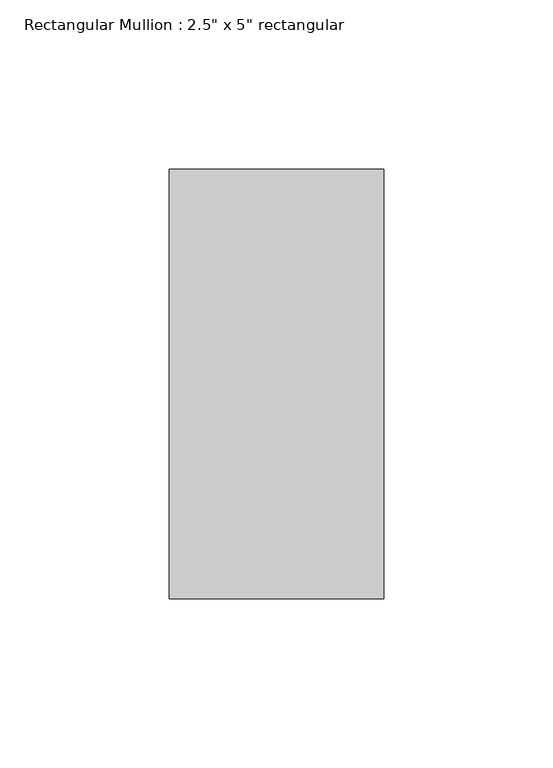
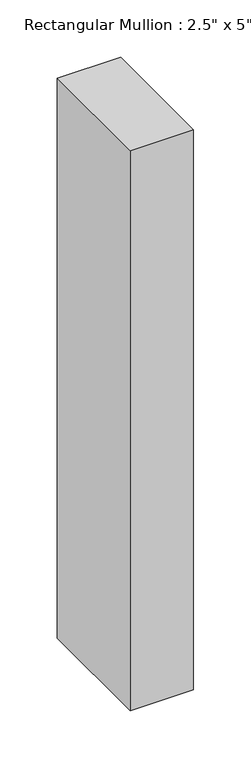
"""IFC4 building model written with IfcOpenShell, lengths in millimetres: member geometry."""

from ifc_helpers import new_model, si_unit, frame, origin, place, context, project, spatial, polyline, outline, extrude, source, transform, mapped, element, save


def member_58197c2e(model_context):
    return source(origin(), model_context, "Body", "SweptSolid", [
        extrude(outline(polyline([(0.0, 63.5), (0.0, -63.5), (-63.5, -63.5), (-63.5, 63.5), (0.0, 63.5)])), frame((0.0, 0.0, -595.5236621), z_axis=(0.0, 0.0, 1.0), x_axis=(1.0, 0.0, 0.0)), (0.0, 0.0, 1.0), 595.5236621),
    ])


if __name__ == "__main__":
    model = new_model("IFC4")
    model_context = context("Model", 3, world=origin())
    ifc_project = project(units=[si_unit("LENGTHUNIT", "METRE", prefix="MILLI")], contexts=[model_context])
    site = spatial("IfcSite", under=ifc_project)
    building = spatial("IfcBuilding", under=site)
    placement = place(None, origin())
    member_shape = member_58197c2e(model_context)
    element("IfcMember", 1, ObjectType="Rectangular Mullion : 2.5\" x 5\" rectangular", at=placement, inside=building, context=model_context, shape_type="MappedRepresentation", body=[
        mapped(member_shape, transform((0.0, 0.0, 0.0), x_axis=(1.0, 0.0, 0.0), y_axis=(0.0, 1.0, 0.0), z_axis=(0.0, 0.0, 1.0))),
    ])
    save(model, "model.ifc")

# Revit data of these elements
# Type "Rectangular Mullion : 2.5\" x 5\" rectangular"
#   built-in parameter 1007304 = 0.416667 (stored number, unit not read)
#   built-in parameter 1007301 = 0.104167 (stored number, unit not read)
#   built-in parameter 1007300 = 0.104167 (stored number, unit not read)
# Element 1 (IfcMember, "Rectangular Mullion : 2.5\" x 5\" rectangular")
#   Materials on its faces: "Aluminum"
# Materials
#   "Aluminum": class "Metal", colour RGB 247 247 247, transparency 0, Description = "Aluminum 6061", Cost = 0
